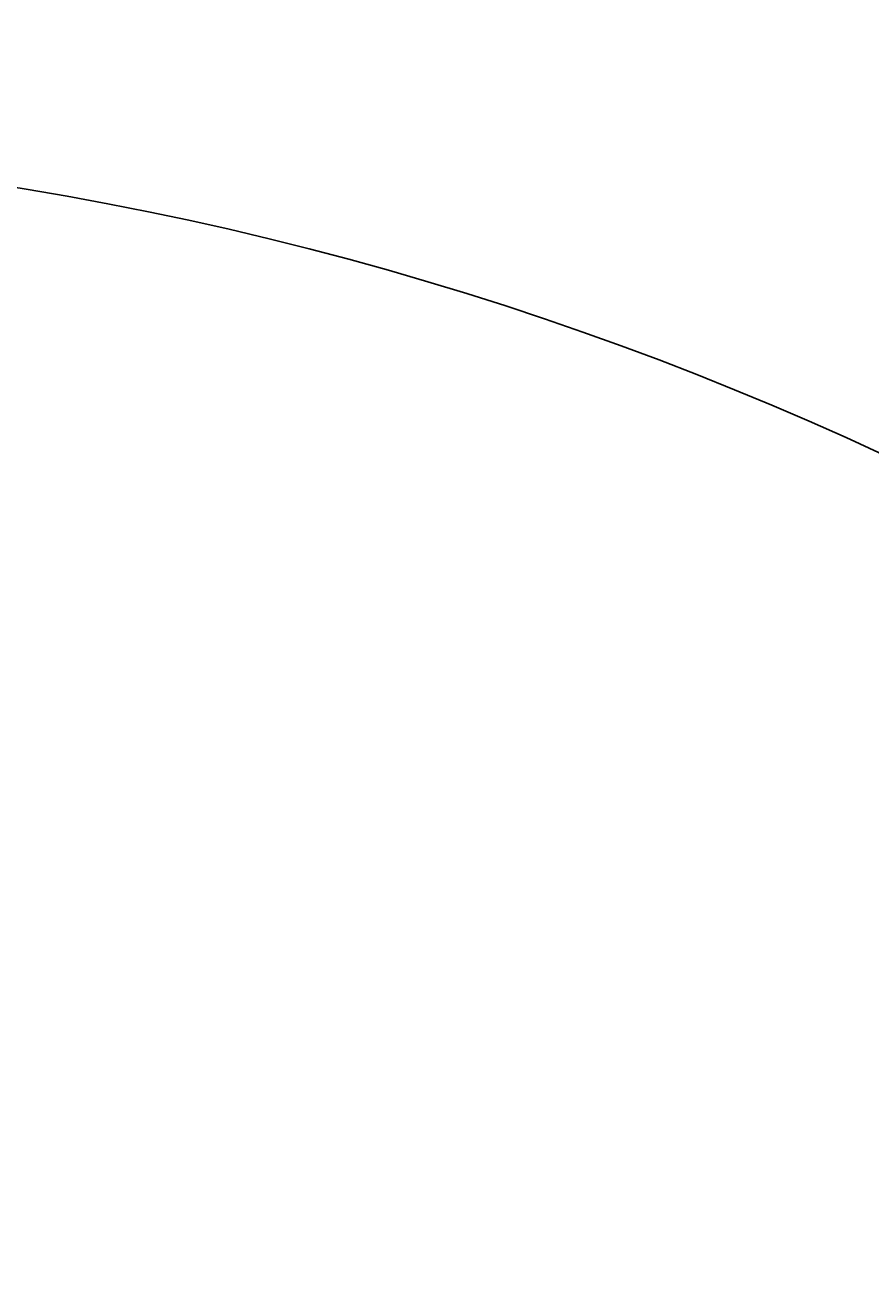
# Model space of a CAD drawing. Units: millimetres. Extents: x 19292 to 100733, y 12374 to 26974.
# Tile 11 of 24: x 29589 to 29777, y 15391 to 15668. Entities that reach past the tile are written whole.
import ezdxf

# ---------------------------------------------------------------- set-up
doc = ezdxf.new("R2010")
doc.units = ezdxf.units.MM
doc.layers.add('A-ANNO-DIMS', color=2, linetype='Continuous', lineweight=18)
doc.layers.add('A-DOOR', color=4, linetype='Continuous', lineweight=25)
doc.styles.get("Standard").update_dxf_attribs({"font": 'arial.ttf'})
doc.dimstyles.get("Standard").update_dxf_attribs({"dimtxt": 0.18, "dimasz": 0.18, "dimexe": 0.18, "dimexo": 0.0625, "dimgap": 0.09, "dimtad": 0, "dimtih": 1, "dimtoh": 1, "dimdec": 4, "dimzin": 0, "dimdsep": 46, "dimtxsty": 'Standard', "dimcen": 0.09, "dimadec": 0, "dimazin": 0, "dimtfac": 1, "dimtdec": 4, "dimtofl": 0, "dimtmove": 0, "dimatfit": 3, "dimfxl": 1, "dimtolj": 1, "dimtzin": 0, "dimarcsym": 0})

# ---------------------------------------------------------------- blocks, each defined once
blk = doc.blocks.new('*D79')
at = {"layer": 'A-ANNO-DIMS', "color": 0, "lineweight": -2, "transparency": 16777216}
for p, q in [((22694.13, 22860.66), (22694.13, 12808.81)), ((36144.17, 15985.66), (36144.17, 12808.81)), ((22694.31, 12808.99), (29418.73, 12808.99)), ((36143.99, 12808.99), (29419.57, 12808.99))]:
    blk.add_line(p, q, dxfattribs=at)
at = {"layer": 'A-ANNO-DIMS', "color": 0, "transparency": 16777216}
for points in [[(22694.31, 12809.02), (22694.31, 12808.96), (22694.13, 12808.99)], [(36143.99, 12809.02), (36143.99, 12808.96), (36144.17, 12808.99)]]:
    blk.add_solid(points, dxfattribs=at)
at = {"layer": 'Defpoints', "color": 0, "transparency": 16777216}
for p in [(22694.13, 22860.72), (36144.17, 15985.72), (36144.17, 12808.99)]:
    blk.add_point(p, dxfattribs=at)
at = {"layer": 'A-ANNO-DIMS', "color": 0, "transparency": 16777216, "insert": (29419.15, 12808.99), "char_height": 0.18, "attachment_point": 5}
blk.add_mtext('\\A1;13450', dxfattribs=at)
blk = doc.blocks.new('*D82')
at = {"layer": 'A-ANNO-DIMS', "color": 0, "lineweight": -2, "transparency": 16777216}
for p, q in [((27198.81, 13562.81), (27198.81, 23555.9)), ((27198.99, 23555.72), (29296.44, 23555.72)), ((31394.62, 23555.72), (29297.17, 23555.72)), ((31394.8, 13544.06), (31394.8, 23555.9))]:
    blk.add_line(p, q, dxfattribs=at)
at = {"layer": 'A-ANNO-DIMS', "color": 0, "transparency": 16777216}
for points in [[(27198.99, 23555.75), (27198.99, 23555.69), (27198.81, 23555.72)], [(31394.62, 23555.75), (31394.62, 23555.69), (31394.8, 23555.72)]]:
    blk.add_solid(points, dxfattribs=at)
at = {"layer": 'Defpoints', "color": 0, "transparency": 16777216}
for p in [(31394.8, 23555.72), (27198.81, 13562.75), (31394.8, 13543.99)]:
    blk.add_point(p, dxfattribs=at)
at = {"layer": 'A-ANNO-DIMS', "color": 0, "transparency": 16777216, "insert": (29296.81, 23555.72), "char_height": 0.18, "attachment_point": 5}
blk.add_mtext('\\A1;4196', dxfattribs=at)
blk = doc.blocks.new('*D86')
at = {"layer": 'A-ANNO-DIMS', "color": 0, "lineweight": -2, "transparency": 16777216}
for p, q in [((27198.81, 15132.81), (27198.81, 23555.9)), ((27198.99, 23555.72), (29198.45, 23555.72)), ((31198.63, 23555.72), (29199.18, 23555.72)), ((31198.81, 15132.81), (31198.81, 23555.9))]:
    blk.add_line(p, q, dxfattribs=at)
at = {"layer": 'A-ANNO-DIMS', "color": 0, "transparency": 16777216}
for points in [[(27198.99, 23555.75), (27198.99, 23555.69), (27198.81, 23555.72)], [(31198.63, 23555.75), (31198.63, 23555.69), (31198.81, 23555.72)]]:
    blk.add_solid(points, dxfattribs=at)
at = {"layer": 'Defpoints', "color": 0, "transparency": 16777216}
for p in [(31198.81, 23555.72), (27198.81, 15132.75), (31198.81, 15132.75)]:
    blk.add_point(p, dxfattribs=at)
at = {"layer": 'A-ANNO-DIMS', "color": 0, "transparency": 16777216, "insert": (29198.81, 23555.72), "char_height": 0.18, "attachment_point": 5}
blk.add_mtext('\\A1;4000', dxfattribs=at)

msp = doc.modelspace()

# ---------------------------------------------------------------- linework, layer by layer
at = {"layer": 'A-DOOR'}
msp.add_arc((29468.571, 14906.403), 735.272, 0, 90, dxfattribs=at)

# ---------------------------------------------------------------- dimensions: what is measured, and where the dimension line sits
at = {"layer": 'A-ANNO-DIMS'}
for base, p1, p2, picture, middle in [((31394.799, 23555.725), (27198.815, 13562.748), (31394.799, 13543.993), '*D82', (29296.807, 23555.725)), ((31198.815, 23555.725), (27198.815, 15132.748), (31198.815, 15132.748), '*D86', (29198.815, 23555.725)), ((36144.169, 12808.993), (22694.132, 22860.725), (36144.169, 15985.725), '*D79', (29419.151, 12808.993))]:
    dim = msp.add_linear_dim(base=base, p1=p1, p2=p2, dimstyle='Standard', override={"dimdec": 0, "dimlfac": 1, "dimrnd": 0, "dimzin": 0, "dimdsep": 46, "dimlunit": 2}, dxfattribs=at)
    dim.commit()
    dim.dimension.update_dxf_attribs({"geometry": picture, "text_midpoint": middle})

doc.saveas('drawing.dxf')
